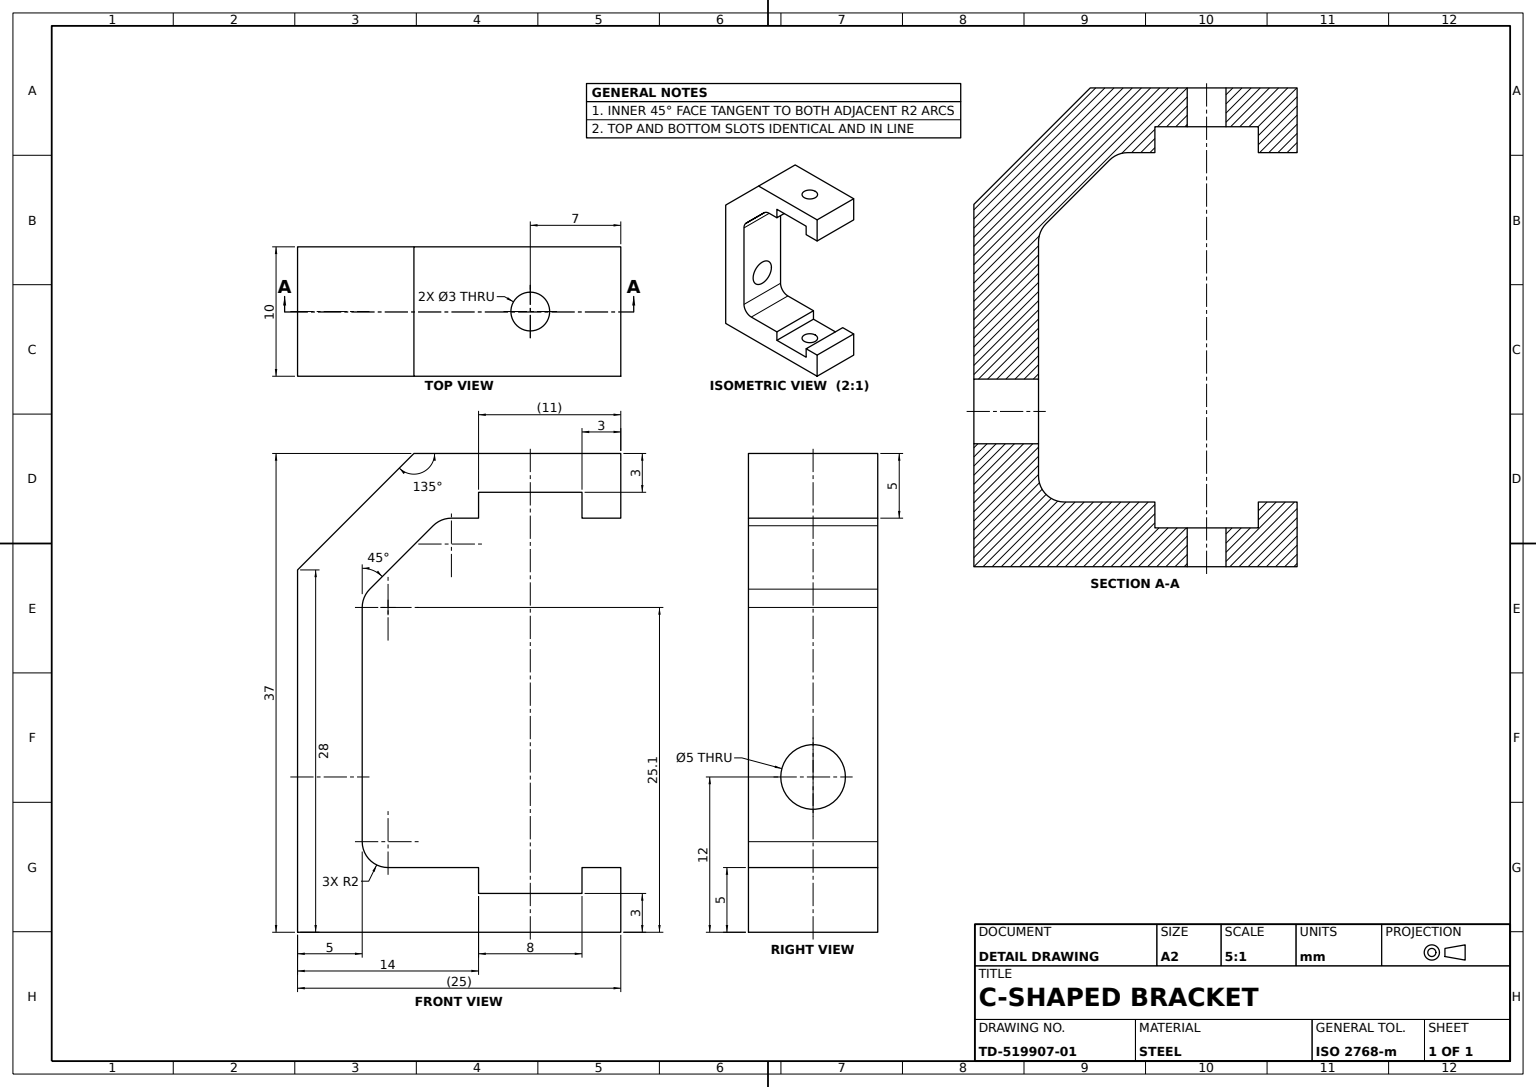
SolidWorks part; units mm, degrees
material "Plain Carbon Steel"
ref_plane "Front Plane" through (0, 0, 0) normal (0, 0, 1) x (1, 0, 0)
ref_plane "Top Plane" through (0, 0, 0) normal (0, 1, 0) x (1, 0, 0)
ref_plane "Right Plane" through (0, 0, 0) normal (1, 0, 0) x (0, 0, -1)
sketch "C Clip Profile Sketch" plane through (0, 0, 0) normal (0, 0, 1) x (1, 0, 0)
  line L0 (0, 0) -> (0, 28)
  line L1 (0, 0) -> (25, 0)
  line L2 (25, 0) -> (25, 5)
  line L3 (25, 5) -> (22, 5)
  line L4 (22, 5) -> (22, 3)
  line L5 (22, 3) -> (14, 3)
  line L6 (14, 3) -> (14, 5)
  line L7 (5, 25.1005) -> (5, 7)
  line L9 (7, 5) -> (14, 5)
  line L10 (0, 28) -> (9, 37)
  line L12 (25, 37) -> (9, 37)
  line L13 (25, 37) -> (25, 32)
  line L14 (25, 32) -> (22, 32)
  line L15 (22, 32) -> (22, 34)
  line L16 (22, 34) -> (14, 34)
  line L17 (14, 34) -> (14, 32)
  line L18 (5.5858, 26.5147) -> (10.4853, 31.4142)
  line L20 (11.8995, 32) -> (14, 32)
  arc A0 (7, 5) -> (5, 7) centre (7, 7) cw
  arc A1 (11.8995, 32) -> (10.4853, 31.4142) centre (11.8995, 30) ccw
  arc A2 (5.5858, 26.5147) -> (5, 25.1005) centre (7, 25.1005) ccw
  dimension "D7" = 2
  dimension "D9" = 2
  dimension "D8" = 2
  dimension "D1" = 28
  dimension "D2" = 25
  dimension "D3" = 5
  dimension "D4" = 3
  dimension "D5" = 2
  dimension "D6" = 8
  dimension "D10" = 45
  dimension "D11" = 37
  dimension "D12" = 5
  dimension "D13" = 3
  dimension "D14" = 2
  dimension "D15" = 8
  dimension "D16" = 2
  dimension "D17" = 18.1005
  dimension "D18" = 13.1005
  dimension "D19" = 29
  dimension "D20" = 4.8995
  dimension "D21" = 18
extrude "C Clip Body" add sketch "C Clip Profile Sketch" along normal blind 10
sketch "Flange Hole 1 Sketch" plane through (0, 3, 0) normal (0, 1, 0) x (1, 0, 0)
  line L0 (25, -10) -> (25, 0) construction
  line L1 (25, -10) -> (9, -10) construction
  circle A0 centre (18, -5) radius 1.5
  dimension "D2" = 3
  dimension "D1" = 7
  dimension "D3" = 5
extrude "Flange Hole 1 Ø3" cut sketch "Flange Hole 1 Sketch" against normal blind 100
sketch "Flange Hole 2 Sketch" plane through (0, 37, 0) normal (0, 1, 0) x (1, 0, 0)
  line L0 (25, -10) -> (25, 0) construction
  line L1 (25, -10) -> (9, -10) construction
  circle A0 centre (18, -5) radius 1.5
  dimension "D1" = 3
  dimension "D2" = 7
  dimension "D3" = 5
extrude "Flange Hole 2 Ø3" cut sketch "Flange Hole 2 Sketch" against normal blind 100
sketch "Web Hole Sketch" plane through (0, 0, 0) normal (-1, 0, 0) x (0, 0, 1)
  line L0 (10, 0) -> (0, 0) construction
  line L1 (0, 28) -> (0, 0) construction
  circle A0 centre (5, 12) radius 2.5
  dimension "D1" = 5
  dimension "D2" = 12
  dimension "D3" = 5
extrude "Web Hole Ø5" cut sketch "Web Hole Sketch" against normal blind 100
